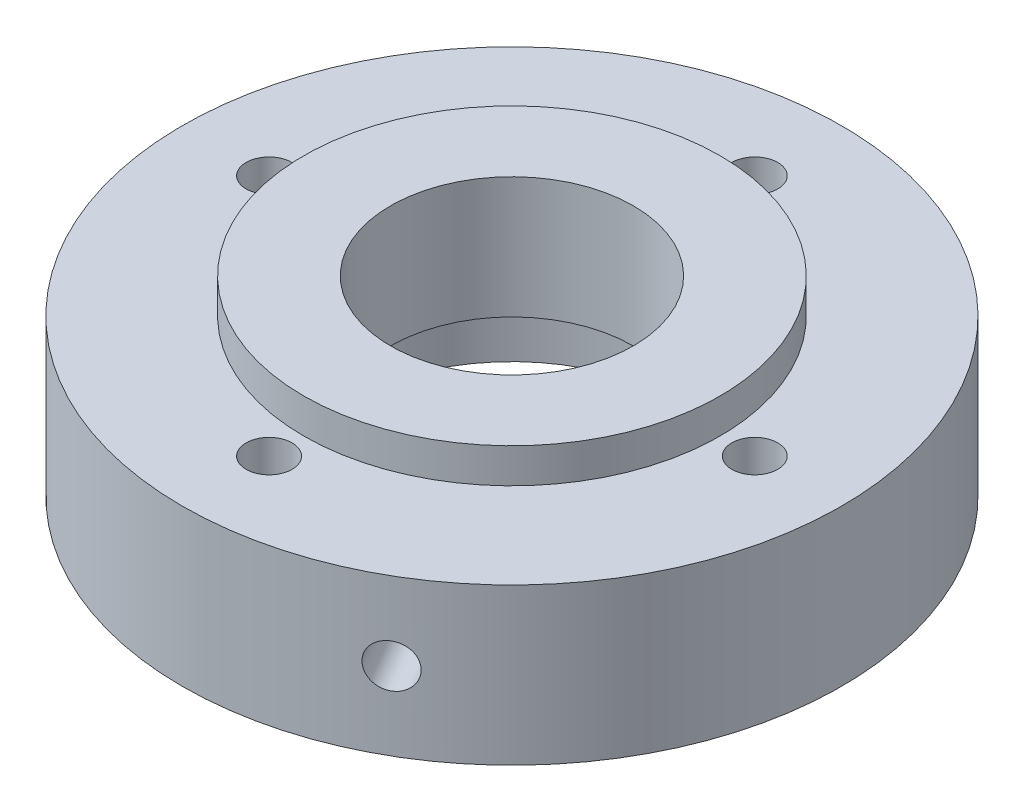
ISO-10303-21;
HEADER;
FILE_DESCRIPTION(('STEP AP214'),'2;1');
FILE_NAME('part.step','',(''),(''),'','','');
FILE_SCHEMA(('AUTOMOTIVE_DESIGN { 1 0 10303 214 1 1 1 1 }'));
ENDSEC;
DATA;
#1=APPLICATION_CONTEXT('core data for automotive mechanical design processes');
#2=APPLICATION_PROTOCOL_DEFINITION('international standard','automotive_design',2000,#1);
#3=PRODUCT_CONTEXT('',#1,'mechanical');
#4=PRODUCT('Part','Part','',(#3));
#5=PRODUCT_RELATED_PRODUCT_CATEGORY('part','',(#4));
#6=PRODUCT_DEFINITION_FORMATION('','',#4);
#7=PRODUCT_DEFINITION_CONTEXT('part definition',#1,'design');
#8=PRODUCT_DEFINITION('design','',#6,#7);
#9=PRODUCT_DEFINITION_SHAPE('','',#8);
#10=(LENGTH_UNIT() NAMED_UNIT(*) SI_UNIT(.MILLI.,.METRE.));
#11=(NAMED_UNIT(*) PLANE_ANGLE_UNIT() SI_UNIT($,.RADIAN.));
#12=(NAMED_UNIT(*) SI_UNIT($,.STERADIAN.) SOLID_ANGLE_UNIT());
#13=UNCERTAINTY_MEASURE_WITH_UNIT(LENGTH_MEASURE(1.E-05),#10,'distance_accuracy_value','');
#14=(GEOMETRIC_REPRESENTATION_CONTEXT(3) GLOBAL_UNCERTAINTY_ASSIGNED_CONTEXT((#13)) GLOBAL_UNIT_ASSIGNED_CONTEXT((#10,
#11,#12)) REPRESENTATION_CONTEXT('',''));
#15=CARTESIAN_POINT('',(0.,0.,0.));
#16=DIRECTION('',(0.,0.,1.));
#17=DIRECTION('',(1.,0.,0.));
#18=AXIS2_PLACEMENT_3D('',#15,#16,#17);
#19=CARTESIAN_POINT('',(0.,9.,0.));
#20=DIRECTION('',(0.,-1.,0.));
#21=DIRECTION('',(0.,0.,-1.));
#22=AXIS2_PLACEMENT_3D('',#19,#20,#21);
#23=CYLINDRICAL_SURFACE('',#22,38.);
#24=CARTESIAN_POINT('',(21.123900499108,0.,31.5876689184844));
#25=CARTESIAN_POINT('',(21.1238957091237,-0.14026296821929,31.587672954066));
#26=CARTESIAN_POINT('',(21.1140367111997,-0.280623770964307,31.594272124677));
#27=CARTESIAN_POINT('',(21.0748168683031,-0.557468570772763,31.6204463654553));
#28=CARTESIAN_POINT('',(21.0454334075926,-0.693947880391754,31.6400364833519));
#29=CARTESIAN_POINT('',(20.967916595861,-0.95897955673141,31.6914598000946));
#30=CARTESIAN_POINT('',(20.9197932437121,-1.08753610842819,31.7232864698813));
#31=CARTESIAN_POINT('',(20.8060316775886,-1.33312465995972,31.7980133802452));
#32=CARTESIAN_POINT('',(20.7403974370897,-1.4501592660541,31.8409111085659));
#33=CARTESIAN_POINT('',(20.5931762627847,-1.66960814521729,31.9363237417059));
#34=CARTESIAN_POINT('',(20.5115662158887,-1.77200085914129,31.9888525733152));
#35=CARTESIAN_POINT('',(20.3345586484823,-1.95907477171309,32.1016621974415));
#36=CARTESIAN_POINT('',(20.2391605494445,-2.0437552268142,32.1619433152218));
#37=CARTESIAN_POINT('',(20.0369910004709,-2.19306785872995,32.288282567244));
#38=CARTESIAN_POINT('',(19.9302094863448,-2.25768209399902,32.3543458041241));
#39=CARTESIAN_POINT('',(19.7082088944471,-2.36491326725031,32.4900509335556));
#40=CARTESIAN_POINT('',(19.5929899149586,-2.40753046141693,32.559692784419));
#41=CARTESIAN_POINT('',(19.3574500570501,-2.46949770266854,32.7002737038991));
#42=CARTESIAN_POINT('',(19.2371368803516,-2.48888166021506,32.7712107281016));
#43=CARTESIAN_POINT('',(18.9946226048038,-2.50393692466989,32.9123683968928));
#44=CARTESIAN_POINT('',(18.8724215291774,-2.49960852303035,32.9825890502759));
#45=CARTESIAN_POINT('',(18.629812232287,-2.46738987486286,33.1202283097107));
#46=CARTESIAN_POINT('',(18.5094015290169,-2.43953610408451,33.1876510841454));
#47=CARTESIAN_POINT('',(18.273667513676,-2.36111400348179,33.3180316189365));
#48=CARTESIAN_POINT('',(18.1583442342758,-2.31054552781078,33.3809893506207));
#49=CARTESIAN_POINT('',(17.9360874792135,-2.18808825789193,33.5009364538799));
#50=CARTESIAN_POINT('',(17.8291605790289,-2.11618296057238,33.5579211592496));
#51=CARTESIAN_POINT('',(17.6269807914162,-1.95310517722637,33.6645604903366));
#52=CARTESIAN_POINT('',(17.531728050049,-1.86193245017493,33.7142150243444));
#53=CARTESIAN_POINT('',(17.3556053972048,-1.6627019182125,33.8052189562838));
#54=CARTESIAN_POINT('',(17.2747630785516,-1.55461244874809,33.8465524403759));
#55=CARTESIAN_POINT('',(17.1301682937497,-1.32472755050962,33.9199636076438));
#56=CARTESIAN_POINT('',(17.0664158352165,-1.20293211562793,33.952041286695));
#57=CARTESIAN_POINT('',(16.957985484699,-0.949072071377019,34.0063291677514));
#58=CARTESIAN_POINT('',(16.9133088240632,-0.817006799736989,34.0285387327707));
#59=CARTESIAN_POINT('',(16.8444496087952,-0.546365405699918,34.0626776289473));
#60=CARTESIAN_POINT('',(16.820266786872,-0.407789368244477,34.0746070941829));
#61=CARTESIAN_POINT('',(16.7931920702844,-0.128338078964031,34.0879587586434));
#62=CARTESIAN_POINT('',(16.7902603680609,0.0125323783636798,34.0894006032779));
#63=CARTESIAN_POINT('',(16.8056762304921,0.292818040330734,34.081803318164));
#64=CARTESIAN_POINT('',(16.8240236722807,0.432233253367982,34.0727642489327));
#65=CARTESIAN_POINT('',(16.881387081484,0.70552541036977,34.0443795985637));
#66=CARTESIAN_POINT('',(16.920384723914,0.839407151357643,34.0250431552276));
#67=CARTESIAN_POINT('',(17.0178070267663,1.09798008966523,33.9764210990002));
#68=CARTESIAN_POINT('',(17.0762318823767,1.22267119462979,33.9471353861469));
#69=CARTESIAN_POINT('',(17.2107892564278,1.45952670684333,33.8791145571879));
#70=CARTESIAN_POINT('',(17.2869479539057,1.57167222814922,33.8403654668937));
#71=CARTESIAN_POINT('',(17.45458149206,1.78006283557162,33.7542062957108));
#72=CARTESIAN_POINT('',(17.5460564984008,1.87630774968148,33.7067961211417));
#73=CARTESIAN_POINT('',(17.7416982345965,2.05031494761945,33.6042309536316));
#74=CARTESIAN_POINT('',(17.8458842859506,2.12804855025184,33.5490641502799));
#75=CARTESIAN_POINT('',(18.0637061593128,2.26263021792935,33.4322863441705));
#76=CARTESIAN_POINT('',(18.1773419179329,2.3194784230582,33.3706753846389));
#77=CARTESIAN_POINT('',(18.4105992907013,2.41062578245923,33.2425557196137));
#78=CARTESIAN_POINT('',(18.5302160183662,2.44494303087561,33.176050992058));
#79=CARTESIAN_POINT('',(18.77202332052,2.49011354081496,33.0398303379182));
#80=CARTESIAN_POINT('',(18.8942138664263,2.50096706276853,32.9701144469845));
#81=CARTESIAN_POINT('',(19.1374242590965,2.49889944252103,32.8295398192453));
#82=CARTESIAN_POINT('',(19.258445880915,2.48602315917565,32.7586834892885));
#83=CARTESIAN_POINT('',(19.4961515734082,2.43695452332046,32.6177738646721));
#84=CARTESIAN_POINT('',(19.6128356366526,2.40076213087149,32.5477205713883));
#85=CARTESIAN_POINT('',(19.8386569858294,2.30609897011035,32.4105716618428));
#86=CARTESIAN_POINT('',(19.9477943666864,2.2476284820792,32.3434760083829));
#87=CARTESIAN_POINT('',(20.1555911399982,2.1100749002662,32.2143931549603));
#88=CARTESIAN_POINT('',(20.2542507892874,2.03099231190029,32.1524058297887));
#89=CARTESIAN_POINT('',(20.4386670176825,1.85429296810048,32.0354936565859));
#90=CARTESIAN_POINT('',(20.5244004228226,1.75664361852911,31.9805815178681));
#91=CARTESIAN_POINT('',(20.6805510807337,1.5456295694054,31.8798285309556));
#92=CARTESIAN_POINT('',(20.7509645857459,1.43226103549673,31.8339899026911));
#93=CARTESIAN_POINT('',(20.8747236923557,1.19288481911541,31.7529747632888));
#94=CARTESIAN_POINT('',(20.9280465194288,1.06686056310857,31.7178124823886));
#95=CARTESIAN_POINT('',(21.0160861318739,0.805961436994182,31.659547325594));
#96=CARTESIAN_POINT('',(21.0508246541216,0.671097114810736,31.6364303618878));
#97=CARTESIAN_POINT('',(21.0918211256234,0.44617637840564,31.6091035052925));
#98=CARTESIAN_POINT('',(21.1038367830818,0.357572910700806,31.6010785819328));
#99=CARTESIAN_POINT('',(21.1198779949323,0.179326293259485,31.5903600025264));
#100=CARTESIAN_POINT('',(21.1239035617899,0.0896831451452361,31.5876663381622));
#101=CARTESIAN_POINT('',(21.123900499108,0.,31.5876689184844));
#102=B_SPLINE_CURVE_WITH_KNOTS('',3,(#24,#25,#26,#27,#28,#29,#30,#31,#32,#33,#34,#35,#36,#37,
#38,#39,#40,#41,#42,#43,#44,#45,#46,#47,#48,#49,#50,#51,#52,#53,#54,#55,#56,#57,#58,#59,#60,#61,
#62,#63,#64,#65,#66,#67,#68,#69,#70,#71,#72,#73,#74,#75,#76,#77,#78,#79,#80,#81,#82,#83,#84,#85,
#86,#87,#88,#89,#90,#91,#92,#93,#94,#95,#96,#97,#98,#99,#100,#101),.UNSPECIFIED.,.T.,.F.,(4,2,2,
2,2,2,2,2,2,2,2,2,2,2,2,2,2,2,2,2,2,2,2,2,2,2,2,2,2,2,2,2,2,2,2,2,2,2,4),(0.,0.420461498480437,
0.841410880410043,1.26213596730298,1.68276566662256,2.10400847286644,2.52526895900485,
2.94690502397213,3.36853617832339,3.78955118149476,4.21056100991944,4.63091926439621,
5.05128021794911,5.47196715304152,5.89265935100819,6.31414862675714,6.7356380903302,
7.15715475706393,7.57866592607824,7.99938731660346,8.42010627789137,8.84045251737814,
9.26080298027826,9.68177795124712,10.1027574758629,10.5243850778361,10.946009851793,
11.3672956121168,11.7885766964458,12.2090622072308,12.6295484382853,13.0500293793716,
13.4705000110872,13.8917157147232,14.3130343462041,14.7349121022704,15.1562953299902,
15.4251358436648,15.6939759379172),.UNSPECIFIED.);
#103=CARTESIAN_POINT('',(21.123900499108,0.,31.5876689184844));
#104=VERTEX_POINT('',#103);
#105=EDGE_CURVE('E70',#104,#104,#102,.T.);
#106=ORIENTED_EDGE('',*,*,#105,.T.);
#107=EDGE_LOOP('',(#106));
#108=FACE_BOUND('',#107,.T.);
#109=CARTESIAN_POINT('',(0.,9.,0.));
#110=DIRECTION('',(0.,1.,0.));
#111=DIRECTION('',(0.,0.,1.));
#112=AXIS2_PLACEMENT_3D('',#109,#110,#111);
#113=CIRCLE('',#112,38.);
#114=CARTESIAN_POINT('',(0.,9.,38.));
#115=VERTEX_POINT('',#114);
#116=EDGE_CURVE('E78',#115,#115,#113,.T.);
#117=ORIENTED_EDGE('',*,*,#116,.F.);
#118=EDGE_LOOP('',(#117));
#119=FACE_BOUND('',#118,.T.);
#120=CARTESIAN_POINT('',(0.,-9.,0.));
#121=DIRECTION('',(0.,1.,0.));
#122=DIRECTION('',(0.,0.,1.));
#123=AXIS2_PLACEMENT_3D('',#120,#121,#122);
#124=CIRCLE('',#123,38.);
#125=CARTESIAN_POINT('',(0.,-9.,38.));
#126=VERTEX_POINT('',#125);
#127=EDGE_CURVE('E81',#126,#126,#124,.T.);
#128=ORIENTED_EDGE('',*,*,#127,.T.);
#129=EDGE_LOOP('',(#128));
#130=FACE_BOUND('',#129,.T.);
#131=ADVANCED_FACE('F39',(#108,#119,#130),#23,.T.);
#132=CARTESIAN_POINT('',(0.,9.,0.));
#133=DIRECTION('',(0.,1.,0.));
#134=DIRECTION('',(0.,0.,1.));
#135=AXIS2_PLACEMENT_3D('',#132,#133,#134);
#136=PLANE('',#135);
#137=CARTESIAN_POINT('',(0.,9.,28.));
#138=DIRECTION('',(0.,-1.,0.));
#139=DIRECTION('',(0.,0.,-1.));
#140=AXIS2_PLACEMENT_3D('',#137,#138,#139);
#141=CIRCLE('',#140,2.65000000000001);
#142=CARTESIAN_POINT('',(0.,9.,25.35));
#143=VERTEX_POINT('',#142);
#144=EDGE_CURVE('E204',#143,#143,#141,.T.);
#145=ORIENTED_EDGE('',*,*,#144,.T.);
#146=EDGE_LOOP('',(#145));
#147=FACE_BOUND('',#146,.T.);
#148=CARTESIAN_POINT('',(28.,9.,0.));
#149=DIRECTION('',(0.,-1.,0.));
#150=DIRECTION('',(0.,0.,-1.));
#151=AXIS2_PLACEMENT_3D('',#148,#149,#150);
#152=CIRCLE('',#151,2.65000000000001);
#153=CARTESIAN_POINT('',(28.,9.,-2.65000000000001));
#154=VERTEX_POINT('',#153);
#155=EDGE_CURVE('E213',#154,#154,#152,.T.);
#156=ORIENTED_EDGE('',*,*,#155,.T.);
#157=EDGE_LOOP('',(#156));
#158=FACE_BOUND('',#157,.T.);
#159=CARTESIAN_POINT('',(0.,9.,-28.));
#160=DIRECTION('',(0.,-1.,0.));
#161=DIRECTION('',(0.,0.,-1.));
#162=AXIS2_PLACEMENT_3D('',#159,#160,#161);
#163=CIRCLE('',#162,2.65000000000001);
#164=CARTESIAN_POINT('',(0.,9.,-30.65));
#165=VERTEX_POINT('',#164);
#166=EDGE_CURVE('E227',#165,#165,#163,.T.);
#167=ORIENTED_EDGE('',*,*,#166,.T.);
#168=EDGE_LOOP('',(#167));
#169=FACE_BOUND('',#168,.T.);
#170=CARTESIAN_POINT('',(-28.,9.,0.));
#171=DIRECTION('',(0.,-1.,0.));
#172=DIRECTION('',(0.,0.,-1.));
#173=AXIS2_PLACEMENT_3D('',#170,#171,#172);
#174=CIRCLE('',#173,2.65000000000001);
#175=CARTESIAN_POINT('',(-28.,9.,-2.65000000000001));
#176=VERTEX_POINT('',#175);
#177=EDGE_CURVE('E237',#176,#176,#174,.T.);
#178=ORIENTED_EDGE('',*,*,#177,.T.);
#179=EDGE_LOOP('',(#178));
#180=FACE_BOUND('',#179,.T.);
#181=CARTESIAN_POINT('',(0.,9.,0.));
#182=DIRECTION('',(0.,1.,0.));
#183=DIRECTION('',(0.,0.,1.));
#184=AXIS2_PLACEMENT_3D('',#181,#182,#183);
#185=CIRCLE('',#184,24.);
#186=CARTESIAN_POINT('',(0.,9.,24.));
#187=VERTEX_POINT('',#186);
#188=EDGE_CURVE('E242',#187,#187,#185,.F.);
#189=ORIENTED_EDGE('',*,*,#188,.T.);
#190=EDGE_LOOP('',(#189));
#191=FACE_BOUND('',#190,.T.);
#192=ORIENTED_EDGE('',*,*,#116,.T.);
#193=EDGE_LOOP('',(#192));
#194=FACE_BOUND('',#193,.T.);
#195=ADVANCED_FACE('F111',(#147,#158,#169,#180,#191,#194),#136,.T.);
#196=CARTESIAN_POINT('',(0.,-9.,0.));
#197=DIRECTION('',(0.,1.,0.));
#198=DIRECTION('',(0.,0.,1.));
#199=AXIS2_PLACEMENT_3D('',#196,#197,#198);
#200=PLANE('',#199);
#201=CARTESIAN_POINT('',(0.,-9.,0.));
#202=DIRECTION('',(0.,1.,0.));
#203=DIRECTION('',(0.,0.,1.));
#204=AXIS2_PLACEMENT_3D('',#201,#202,#203);
#205=CIRCLE('',#204,19.);
#206=CARTESIAN_POINT('',(0.,-9.,19.));
#207=VERTEX_POINT('',#206);
#208=EDGE_CURVE('E86',#207,#207,#205,.T.);
#209=ORIENTED_EDGE('',*,*,#208,.T.);
#210=EDGE_LOOP('',(#209));
#211=FACE_BOUND('',#210,.T.);
#212=CARTESIAN_POINT('',(0.,-9.,28.));
#213=DIRECTION('',(0.,-1.,0.));
#214=DIRECTION('',(0.,0.,-1.));
#215=AXIS2_PLACEMENT_3D('',#212,#213,#214);
#216=CIRCLE('',#215,3.90000000000001);
#217=CARTESIAN_POINT('',(0.,-9.,24.1));
#218=VERTEX_POINT('',#217);
#219=EDGE_CURVE('E194',#218,#218,#216,.T.);
#220=ORIENTED_EDGE('',*,*,#219,.F.);
#221=EDGE_LOOP('',(#220));
#222=FACE_BOUND('',#221,.T.);
#223=CARTESIAN_POINT('',(28.,-9.,0.));
#224=DIRECTION('',(0.,-1.,0.));
#225=DIRECTION('',(0.,0.,-1.));
#226=AXIS2_PLACEMENT_3D('',#223,#224,#225);
#227=CIRCLE('',#226,3.90000000000001);
#228=CARTESIAN_POINT('',(28.,-9.,-3.90000000000001));
#229=VERTEX_POINT('',#228);
#230=EDGE_CURVE('E207',#229,#229,#227,.T.);
#231=ORIENTED_EDGE('',*,*,#230,.F.);
#232=EDGE_LOOP('',(#231));
#233=FACE_BOUND('',#232,.T.);
#234=CARTESIAN_POINT('',(0.,-9.,-28.));
#235=DIRECTION('',(0.,-1.,0.));
#236=DIRECTION('',(0.,0.,-1.));
#237=AXIS2_PLACEMENT_3D('',#234,#235,#236);
#238=CIRCLE('',#237,3.90000000000001);
#239=CARTESIAN_POINT('',(0.,-9.,-31.9));
#240=VERTEX_POINT('',#239);
#241=EDGE_CURVE('E220',#240,#240,#238,.T.);
#242=ORIENTED_EDGE('',*,*,#241,.F.);
#243=EDGE_LOOP('',(#242));
#244=FACE_BOUND('',#243,.T.);
#245=CARTESIAN_POINT('',(-28.,-9.,0.));
#246=DIRECTION('',(0.,-1.,0.));
#247=DIRECTION('',(0.,0.,-1.));
#248=AXIS2_PLACEMENT_3D('',#245,#246,#247);
#249=CIRCLE('',#248,3.90000000000001);
#250=CARTESIAN_POINT('',(-28.,-9.,-3.90000000000001));
#251=VERTEX_POINT('',#250);
#252=EDGE_CURVE('E229',#251,#251,#249,.T.);
#253=ORIENTED_EDGE('',*,*,#252,.F.);
#254=EDGE_LOOP('',(#253));
#255=FACE_BOUND('',#254,.T.);
#256=ORIENTED_EDGE('',*,*,#127,.F.);
#257=EDGE_LOOP('',(#256));
#258=FACE_BOUND('',#257,.T.);
#259=ADVANCED_FACE('F113',(#211,#222,#233,#244,#255,#258),#200,.F.);
#260=CARTESIAN_POINT('',(0.,13.,0.));
#261=DIRECTION('',(0.,-1.,0.));
#262=DIRECTION('',(0.,0.,-1.));
#263=AXIS2_PLACEMENT_3D('',#260,#261,#262);
#264=CYLINDRICAL_SURFACE('',#263,24.);
#265=ORIENTED_EDGE('',*,*,#188,.F.);
#266=EDGE_LOOP('',(#265));
#267=FACE_BOUND('',#266,.T.);
#268=CARTESIAN_POINT('',(0.,13.,0.));
#269=DIRECTION('',(0.,1.,0.));
#270=DIRECTION('',(0.,0.,1.));
#271=AXIS2_PLACEMENT_3D('',#268,#269,#270);
#272=CIRCLE('',#271,24.);
#273=CARTESIAN_POINT('',(0.,13.,24.));
#274=VERTEX_POINT('',#273);
#275=EDGE_CURVE('E245',#274,#274,#272,.T.);
#276=ORIENTED_EDGE('',*,*,#275,.F.);
#277=EDGE_LOOP('',(#276));
#278=FACE_BOUND('',#277,.T.);
#279=ADVANCED_FACE('F116',(#267,#278),#264,.T.);
#280=CARTESIAN_POINT('',(0.,13.,0.));
#281=DIRECTION('',(0.,1.,0.));
#282=DIRECTION('',(0.,0.,1.));
#283=AXIS2_PLACEMENT_3D('',#280,#281,#282);
#284=PLANE('',#283);
#285=CARTESIAN_POINT('',(0.,13.,0.));
#286=DIRECTION('',(0.,1.,0.));
#287=DIRECTION('',(0.,0.,1.));
#288=AXIS2_PLACEMENT_3D('',#285,#286,#287);
#289=CIRCLE('',#288,14.);
#290=CARTESIAN_POINT('',(0.,13.,-14.));
#291=VERTEX_POINT('',#290);
#292=EDGE_CURVE('E102',#291,#291,#289,.F.);
#293=ORIENTED_EDGE('',*,*,#292,.T.);
#294=EDGE_LOOP('',(#293));
#295=FACE_BOUND('',#294,.T.);
#296=ORIENTED_EDGE('',*,*,#275,.T.);
#297=EDGE_LOOP('',(#296));
#298=FACE_BOUND('',#297,.T.);
#299=ADVANCED_FACE('F124',(#295,#298),#284,.T.);
#300=CARTESIAN_POINT('',(-28.,-9.,0.));
#301=DIRECTION('',(0.,-1.,0.));
#302=DIRECTION('',(0.,0.,-1.));
#303=AXIS2_PLACEMENT_3D('',#300,#301,#302);
#304=CYLINDRICAL_SURFACE('',#303,2.65000000000001);
#305=ORIENTED_EDGE('',*,*,#177,.F.);
#306=EDGE_LOOP('',(#305));
#307=FACE_BOUND('',#306,.T.);
#308=CARTESIAN_POINT('',(-28.,-5.,0.));
#309=DIRECTION('',(0.,-1.,0.));
#310=DIRECTION('',(0.,0.,-1.));
#311=AXIS2_PLACEMENT_3D('',#308,#309,#310);
#312=CIRCLE('',#311,2.65000000000001);
#313=CARTESIAN_POINT('',(-28.,-5.,-2.65000000000001));
#314=VERTEX_POINT('',#313);
#315=EDGE_CURVE('E236',#314,#314,#312,.T.);
#316=ORIENTED_EDGE('',*,*,#315,.T.);
#317=EDGE_LOOP('',(#316));
#318=FACE_BOUND('',#317,.T.);
#319=ADVANCED_FACE('F130',(#307,#318),#304,.F.);
#320=CARTESIAN_POINT('',(-25.35,-5.,0.));
#321=DIRECTION('',(0.,1.,0.));
#322=DIRECTION('',(0.,0.,1.));
#323=AXIS2_PLACEMENT_3D('',#320,#321,#322);
#324=PLANE('',#323);
#325=ORIENTED_EDGE('',*,*,#315,.F.);
#326=EDGE_LOOP('',(#325));
#327=FACE_BOUND('',#326,.T.);
#328=CARTESIAN_POINT('',(-28.,-5.,0.));
#329=DIRECTION('',(0.,-1.,0.));
#330=DIRECTION('',(0.,0.,-1.));
#331=AXIS2_PLACEMENT_3D('',#328,#329,#330);
#332=CIRCLE('',#331,3.90000000000001);
#333=CARTESIAN_POINT('',(-28.,-5.,-3.90000000000001));
#334=VERTEX_POINT('',#333);
#335=EDGE_CURVE('E231',#334,#334,#332,.T.);
#336=ORIENTED_EDGE('',*,*,#335,.T.);
#337=EDGE_LOOP('',(#336));
#338=FACE_BOUND('',#337,.T.);
#339=ADVANCED_FACE('F134',(#327,#338),#324,.F.);
#340=CARTESIAN_POINT('',(-28.,-9.,0.));
#341=DIRECTION('',(0.,-1.,0.));
#342=DIRECTION('',(0.,0.,-1.));
#343=AXIS2_PLACEMENT_3D('',#340,#341,#342);
#344=CYLINDRICAL_SURFACE('',#343,3.90000000000001);
#345=ORIENTED_EDGE('',*,*,#335,.F.);
#346=EDGE_LOOP('',(#345));
#347=FACE_BOUND('',#346,.T.);
#348=ORIENTED_EDGE('',*,*,#252,.T.);
#349=EDGE_LOOP('',(#348));
#350=FACE_BOUND('',#349,.T.);
#351=ADVANCED_FACE('F132',(#347,#350),#344,.F.);
#352=CARTESIAN_POINT('',(0.,-9.,-28.));
#353=DIRECTION('',(0.,-1.,0.));
#354=DIRECTION('',(0.,0.,-1.));
#355=AXIS2_PLACEMENT_3D('',#352,#353,#354);
#356=CYLINDRICAL_SURFACE('',#355,2.65000000000001);
#357=ORIENTED_EDGE('',*,*,#166,.F.);
#358=EDGE_LOOP('',(#357));
#359=FACE_BOUND('',#358,.T.);
#360=CARTESIAN_POINT('',(0.,-5.,-28.));
#361=DIRECTION('',(0.,-1.,0.));
#362=DIRECTION('',(0.,0.,-1.));
#363=AXIS2_PLACEMENT_3D('',#360,#361,#362);
#364=CIRCLE('',#363,2.65000000000001);
#365=CARTESIAN_POINT('',(0.,-5.,-30.65));
#366=VERTEX_POINT('',#365);
#367=EDGE_CURVE('E221',#366,#366,#364,.T.);
#368=ORIENTED_EDGE('',*,*,#367,.T.);
#369=EDGE_LOOP('',(#368));
#370=FACE_BOUND('',#369,.T.);
#371=ADVANCED_FACE('F136',(#359,#370),#356,.F.);
#372=CARTESIAN_POINT('',(2.65000000000001,-5.,-28.));
#373=DIRECTION('',(0.,1.,0.));
#374=DIRECTION('',(0.,0.,1.));
#375=AXIS2_PLACEMENT_3D('',#372,#373,#374);
#376=PLANE('',#375);
#377=ORIENTED_EDGE('',*,*,#367,.F.);
#378=EDGE_LOOP('',(#377));
#379=FACE_BOUND('',#378,.T.);
#380=CARTESIAN_POINT('',(0.,-5.,-28.));
#381=DIRECTION('',(0.,-1.,0.));
#382=DIRECTION('',(0.,0.,-1.));
#383=AXIS2_PLACEMENT_3D('',#380,#381,#382);
#384=CIRCLE('',#383,3.90000000000001);
#385=CARTESIAN_POINT('',(0.,-5.,-31.9));
#386=VERTEX_POINT('',#385);
#387=EDGE_CURVE('E222',#386,#386,#384,.T.);
#388=ORIENTED_EDGE('',*,*,#387,.T.);
#389=EDGE_LOOP('',(#388));
#390=FACE_BOUND('',#389,.T.);
#391=ADVANCED_FACE('F141',(#379,#390),#376,.F.);
#392=CARTESIAN_POINT('',(0.,-9.,-28.));
#393=DIRECTION('',(0.,-1.,0.));
#394=DIRECTION('',(0.,0.,-1.));
#395=AXIS2_PLACEMENT_3D('',#392,#393,#394);
#396=CYLINDRICAL_SURFACE('',#395,3.90000000000001);
#397=ORIENTED_EDGE('',*,*,#387,.F.);
#398=EDGE_LOOP('',(#397));
#399=FACE_BOUND('',#398,.T.);
#400=ORIENTED_EDGE('',*,*,#241,.T.);
#401=EDGE_LOOP('',(#400));
#402=FACE_BOUND('',#401,.T.);
#403=ADVANCED_FACE('F150',(#399,#402),#396,.F.);
#404=CARTESIAN_POINT('',(28.,-9.,0.));
#405=DIRECTION('',(0.,-1.,0.));
#406=DIRECTION('',(0.,0.,-1.));
#407=AXIS2_PLACEMENT_3D('',#404,#405,#406);
#408=CYLINDRICAL_SURFACE('',#407,2.65000000000001);
#409=ORIENTED_EDGE('',*,*,#155,.F.);
#410=EDGE_LOOP('',(#409));
#411=FACE_BOUND('',#410,.T.);
#412=CARTESIAN_POINT('',(28.,-5.,0.));
#413=DIRECTION('',(0.,-1.,0.));
#414=DIRECTION('',(0.,0.,-1.));
#415=AXIS2_PLACEMENT_3D('',#412,#413,#414);
#416=CIRCLE('',#415,2.65000000000001);
#417=CARTESIAN_POINT('',(28.,-5.,-2.65000000000001));
#418=VERTEX_POINT('',#417);
#419=EDGE_CURVE('E215',#418,#418,#416,.T.);
#420=ORIENTED_EDGE('',*,*,#419,.T.);
#421=EDGE_LOOP('',(#420));
#422=FACE_BOUND('',#421,.T.);
#423=ADVANCED_FACE('F154',(#411,#422),#408,.F.);
#424=CARTESIAN_POINT('',(30.65,-5.,0.));
#425=DIRECTION('',(0.,1.,0.));
#426=DIRECTION('',(0.,0.,1.));
#427=AXIS2_PLACEMENT_3D('',#424,#425,#426);
#428=PLANE('',#427);
#429=ORIENTED_EDGE('',*,*,#419,.F.);
#430=EDGE_LOOP('',(#429));
#431=FACE_BOUND('',#430,.T.);
#432=CARTESIAN_POINT('',(28.,-5.,0.));
#433=DIRECTION('',(0.,-1.,0.));
#434=DIRECTION('',(0.,0.,-1.));
#435=AXIS2_PLACEMENT_3D('',#432,#433,#434);
#436=CIRCLE('',#435,3.90000000000001);
#437=CARTESIAN_POINT('',(28.,-5.,-3.90000000000001));
#438=VERTEX_POINT('',#437);
#439=EDGE_CURVE('E209',#438,#438,#436,.T.);
#440=ORIENTED_EDGE('',*,*,#439,.T.);
#441=EDGE_LOOP('',(#440));
#442=FACE_BOUND('',#441,.T.);
#443=ADVANCED_FACE('F152',(#431,#442),#428,.F.);
#444=CARTESIAN_POINT('',(28.,-9.,0.));
#445=DIRECTION('',(0.,-1.,0.));
#446=DIRECTION('',(0.,0.,-1.));
#447=AXIS2_PLACEMENT_3D('',#444,#445,#446);
#448=CYLINDRICAL_SURFACE('',#447,3.90000000000001);
#449=ORIENTED_EDGE('',*,*,#439,.F.);
#450=EDGE_LOOP('',(#449));
#451=FACE_BOUND('',#450,.T.);
#452=ORIENTED_EDGE('',*,*,#230,.T.);
#453=EDGE_LOOP('',(#452));
#454=FACE_BOUND('',#453,.T.);
#455=ADVANCED_FACE('F156',(#451,#454),#448,.F.);
#456=CARTESIAN_POINT('',(0.,-9.,28.));
#457=DIRECTION('',(0.,-1.,0.));
#458=DIRECTION('',(0.,0.,-1.));
#459=AXIS2_PLACEMENT_3D('',#456,#457,#458);
#460=CYLINDRICAL_SURFACE('',#459,2.65000000000001);
#461=ORIENTED_EDGE('',*,*,#144,.F.);
#462=EDGE_LOOP('',(#461));
#463=FACE_BOUND('',#462,.T.);
#464=CARTESIAN_POINT('',(0.,-5.,28.));
#465=DIRECTION('',(0.,-1.,0.));
#466=DIRECTION('',(0.,0.,-1.));
#467=AXIS2_PLACEMENT_3D('',#464,#465,#466);
#468=CIRCLE('',#467,2.65000000000001);
#469=CARTESIAN_POINT('',(0.,-5.,25.35));
#470=VERTEX_POINT('',#469);
#471=EDGE_CURVE('E197',#470,#470,#468,.T.);
#472=ORIENTED_EDGE('',*,*,#471,.T.);
#473=EDGE_LOOP('',(#472));
#474=FACE_BOUND('',#473,.T.);
#475=ADVANCED_FACE('F161',(#463,#474),#460,.F.);
#476=CARTESIAN_POINT('',(2.65000000000001,-5.,28.));
#477=DIRECTION('',(0.,1.,0.));
#478=DIRECTION('',(0.,0.,1.));
#479=AXIS2_PLACEMENT_3D('',#476,#477,#478);
#480=PLANE('',#479);
#481=ORIENTED_EDGE('',*,*,#471,.F.);
#482=EDGE_LOOP('',(#481));
#483=FACE_BOUND('',#482,.T.);
#484=CARTESIAN_POINT('',(0.,-5.,28.));
#485=DIRECTION('',(0.,-1.,0.));
#486=DIRECTION('',(0.,0.,-1.));
#487=AXIS2_PLACEMENT_3D('',#484,#485,#486);
#488=CIRCLE('',#487,3.90000000000001);
#489=CARTESIAN_POINT('',(0.,-5.,24.1));
#490=VERTEX_POINT('',#489);
#491=EDGE_CURVE('E196',#490,#490,#488,.T.);
#492=ORIENTED_EDGE('',*,*,#491,.T.);
#493=EDGE_LOOP('',(#492));
#494=FACE_BOUND('',#493,.T.);
#495=ADVANCED_FACE('F170',(#483,#494),#480,.F.);
#496=CARTESIAN_POINT('',(0.,-9.,28.));
#497=DIRECTION('',(0.,-1.,0.));
#498=DIRECTION('',(0.,0.,-1.));
#499=AXIS2_PLACEMENT_3D('',#496,#497,#498);
#500=CYLINDRICAL_SURFACE('',#499,3.90000000000001);
#501=ORIENTED_EDGE('',*,*,#491,.F.);
#502=EDGE_LOOP('',(#501));
#503=FACE_BOUND('',#502,.T.);
#504=ORIENTED_EDGE('',*,*,#219,.T.);
#505=EDGE_LOOP('',(#504));
#506=FACE_BOUND('',#505,.T.);
#507=ADVANCED_FACE('F171',(#503,#506),#500,.F.);
#508=CARTESIAN_POINT('',(0.,-1.,0.));
#509=DIRECTION('',(0.,-1.,0.));
#510=DIRECTION('',(0.,0.,-1.));
#511=AXIS2_PLACEMENT_3D('',#508,#509,#510);
#512=CYLINDRICAL_SURFACE('',#511,19.);
#513=CARTESIAN_POINT('',(0.,-3.,0.));
#514=DIRECTION('',(0.,-1.,0.));
#515=DIRECTION('',(0.,0.,-1.));
#516=AXIS2_PLACEMENT_3D('',#513,#514,#515);
#517=CIRCLE('',#516,19.);
#518=CARTESIAN_POINT('',(0.,-3.,-19.));
#519=VERTEX_POINT('',#518);
#520=EDGE_CURVE('E63',#519,#519,#517,.F.);
#521=ORIENTED_EDGE('',*,*,#520,.T.);
#522=EDGE_LOOP('',(#521));
#523=FACE_BOUND('',#522,.T.);
#524=ORIENTED_EDGE('',*,*,#208,.F.);
#525=EDGE_LOOP('',(#524));
#526=FACE_BOUND('',#525,.T.);
#527=ADVANCED_FACE('F174',(#523,#526),#512,.F.);
#528=CARTESIAN_POINT('',(0.,-1.,0.));
#529=DIRECTION('',(0.,-1.,0.));
#530=DIRECTION('',(0.,0.,-1.));
#531=AXIS2_PLACEMENT_3D('',#528,#529,#530);
#532=PLANE('',#531);
#533=CARTESIAN_POINT('',(0.,-1.,0.));
#534=DIRECTION('',(0.,-1.,0.));
#535=DIRECTION('',(0.,0.,-1.));
#536=AXIS2_PLACEMENT_3D('',#533,#534,#535);
#537=CIRCLE('',#536,17.);
#538=CARTESIAN_POINT('',(0.,-1.,-17.));
#539=VERTEX_POINT('',#538);
#540=EDGE_CURVE('E76',#539,#539,#537,.T.);
#541=ORIENTED_EDGE('',*,*,#540,.T.);
#542=EDGE_LOOP('',(#541));
#543=FACE_BOUND('',#542,.T.);
#544=CARTESIAN_POINT('',(0.,-1.,0.));
#545=DIRECTION('',(0.,-1.,0.));
#546=DIRECTION('',(0.,0.,-1.));
#547=AXIS2_PLACEMENT_3D('',#544,#545,#546);
#548=CIRCLE('',#547,14.);
#549=CARTESIAN_POINT('',(0.,-0.999999999999999,-14.));
#550=VERTEX_POINT('',#549);
#551=EDGE_CURVE('E106',#550,#550,#548,.T.);
#552=ORIENTED_EDGE('',*,*,#551,.F.);
#553=EDGE_LOOP('',(#552));
#554=FACE_BOUND('',#553,.T.);
#555=ADVANCED_FACE('F177',(#543,#554),#532,.T.);
#556=CARTESIAN_POINT('',(0.,13.001,0.));
#557=DIRECTION('',(0.,-1.,0.));
#558=DIRECTION('',(0.,0.,-1.));
#559=AXIS2_PLACEMENT_3D('',#556,#557,#558);
#560=CYLINDRICAL_SURFACE('',#559,14.);
#561=CARTESIAN_POINT('',(0.,13.,-14.));
#562=CARTESIAN_POINT('',(0.,12.8541666666667,-14.));
#563=CARTESIAN_POINT('',(0.,12.7083333333333,-14.));
#564=CARTESIAN_POINT('',(0.,12.4166666666667,-14.));
#565=CARTESIAN_POINT('',(0.,12.2708333333333,-14.));
#566=CARTESIAN_POINT('',(0.,11.9791666666667,-14.));
#567=CARTESIAN_POINT('',(0.,11.8333333333333,-14.));
#568=CARTESIAN_POINT('',(0.,11.5416666666667,-14.));
#569=CARTESIAN_POINT('',(0.,11.3958333333333,-14.));
#570=CARTESIAN_POINT('',(0.,11.1041666666667,-14.));
#571=CARTESIAN_POINT('',(0.,10.9583333333333,-14.));
#572=CARTESIAN_POINT('',(0.,10.6666666666667,-14.));
#573=CARTESIAN_POINT('',(0.,10.5208333333333,-14.));
#574=CARTESIAN_POINT('',(0.,10.2291666666667,-14.));
#575=CARTESIAN_POINT('',(0.,10.0833333333333,-14.));
#576=CARTESIAN_POINT('',(0.,9.79166666666667,-14.));
#577=CARTESIAN_POINT('',(0.,9.64583333333333,-14.));
#578=CARTESIAN_POINT('',(0.,9.35416666666667,-14.));
#579=CARTESIAN_POINT('',(0.,9.20833333333333,-14.));
#580=CARTESIAN_POINT('',(0.,8.91666666666667,-14.));
#581=CARTESIAN_POINT('',(0.,8.77083333333333,-14.));
#582=CARTESIAN_POINT('',(0.,8.47916666666667,-14.));
#583=CARTESIAN_POINT('',(0.,8.33333333333333,-14.));
#584=CARTESIAN_POINT('',(0.,8.04166666666667,-14.));
#585=CARTESIAN_POINT('',(0.,7.89583333333333,-14.));
#586=CARTESIAN_POINT('',(0.,7.60416666666667,-14.));
#587=CARTESIAN_POINT('',(0.,7.45833333333333,-14.));
#588=CARTESIAN_POINT('',(0.,7.16666666666667,-14.));
#589=CARTESIAN_POINT('',(0.,7.02083333333333,-14.));
#590=CARTESIAN_POINT('',(0.,6.72916666666667,-14.));
#591=CARTESIAN_POINT('',(0.,6.58333333333333,-14.));
#592=CARTESIAN_POINT('',(0.,6.29166666666667,-14.));
#593=CARTESIAN_POINT('',(0.,6.14583333333333,-14.));
#594=CARTESIAN_POINT('',(0.,5.85416666666667,-14.));
#595=CARTESIAN_POINT('',(0.,5.70833333333333,-14.));
#596=CARTESIAN_POINT('',(0.,5.41666666666667,-14.));
#597=CARTESIAN_POINT('',(0.,5.27083333333333,-14.));
#598=CARTESIAN_POINT('',(0.,4.97916666666667,-14.));
#599=CARTESIAN_POINT('',(0.,4.83333333333333,-14.));
#600=CARTESIAN_POINT('',(0.,4.54166666666667,-14.));
#601=CARTESIAN_POINT('',(0.,4.39583333333334,-14.));
#602=CARTESIAN_POINT('',(0.,4.10416666666667,-14.));
#603=CARTESIAN_POINT('',(0.,3.95833333333334,-14.));
#604=CARTESIAN_POINT('',(0.,3.66666666666667,-14.));
#605=CARTESIAN_POINT('',(0.,3.52083333333333,-14.));
#606=CARTESIAN_POINT('',(0.,3.22916666666667,-14.));
#607=CARTESIAN_POINT('',(0.,3.08333333333333,-14.));
#608=CARTESIAN_POINT('',(0.,2.79166666666667,-14.));
#609=CARTESIAN_POINT('',(0.,2.64583333333333,-14.));
#610=CARTESIAN_POINT('',(0.,2.35416666666667,-14.));
#611=CARTESIAN_POINT('',(0.,2.20833333333333,-14.));
#612=CARTESIAN_POINT('',(0.,1.91666666666667,-14.));
#613=CARTESIAN_POINT('',(0.,1.77083333333333,-14.));
#614=CARTESIAN_POINT('',(0.,1.47916666666667,-14.));
#615=CARTESIAN_POINT('',(0.,1.33333333333334,-14.));
#616=CARTESIAN_POINT('',(0.,1.04166666666667,-14.));
#617=CARTESIAN_POINT('',(0.,0.895833333333336,-14.));
#618=CARTESIAN_POINT('',(0.,0.604166666666669,-14.));
#619=CARTESIAN_POINT('',(0.,0.458333333333335,-14.));
#620=CARTESIAN_POINT('',(0.,0.166666666666669,-14.));
#621=CARTESIAN_POINT('',(0.,0.020833333333335,-14.));
#622=CARTESIAN_POINT('',(0.,-0.270833333333332,-14.));
#623=CARTESIAN_POINT('',(0.,-0.416666666666665,-14.));
#624=CARTESIAN_POINT('',(0.,-0.708333333333332,-14.));
#625=CARTESIAN_POINT('',(0.,-0.854166666666666,-14.));
#626=CARTESIAN_POINT('',(0.,-0.999999999999999,-14.));
#627=B_SPLINE_CURVE_WITH_KNOTS('',3,(#561,#562,#563,#564,#565,#566,#567,#568,#569,#570,#571,
#572,#573,#574,#575,#576,#577,#578,#579,#580,#581,#582,#583,#584,#585,#586,#587,#588,#589,#590,
#591,#592,#593,#594,#595,#596,#597,#598,#599,#600,#601,#602,#603,#604,#605,#606,#607,#608,#609,
#610,#611,#612,#613,#614,#615,#616,#617,#618,#619,#620,#621,#622,#623,#624,#625,#626),
.UNSPECIFIED.,.F.,.F.,(4,2,2,2,2,2,2,2,2,2,2,2,2,2,2,2,2,2,2,2,2,2,2,2,2,2,2,2,2,2,2,2,4),(0.,
0.4375,0.875000000000001,1.3125,1.75,2.1875,2.625,3.0625,3.5,3.9375,4.375,4.8125,5.25,5.6875,
6.125,6.5625,7.,7.4375,7.875,8.3125,8.75,9.1875,9.625,10.0625,10.5,10.9375,11.375,11.8125,12.25,
12.6875,13.125,13.5625,14.),.UNSPECIFIED.);
#628=EDGE_CURVE('BSEAM75',#291,#550,#627,.T.);
#629=ORIENTED_EDGE('',*,*,#292,.F.);
#630=ORIENTED_EDGE('',*,*,#551,.T.);
#631=ORIENTED_EDGE('',*,*,#628,.T.);
#632=ORIENTED_EDGE('',*,*,#628,.F.);
#633=EDGE_LOOP('',(#629,#631,#630,#632));
#634=FACE_BOUND('',#633,.T.);
#635=ADVANCED_FACE('F75',(#634),#560,.F.);
#636=CARTESIAN_POINT('',(0.,-3.,0.));
#637=DIRECTION('',(0.,-1.,0.));
#638=DIRECTION('',(0.,0.,-1.));
#639=AXIS2_PLACEMENT_3D('',#636,#637,#638);
#640=TOROIDAL_SURFACE('',#639,17.,2.);
#641=CARTESIAN_POINT('',(6.83473649053892,-1.1200623540004,16.3082161467188));
#642=CARTESIAN_POINT('',(6.86691117170615,-1.13740193652086,16.346550439636));
#643=CARTESIAN_POINT('',(6.89964418960741,-1.15648925399527,16.3836245638145));
#644=CARTESIAN_POINT('',(6.96625212535524,-1.19782630817378,16.4548751967557));
#645=CARTESIAN_POINT('',(7.0001271144858,-1.22007624257424,16.4890515241628));
#646=CARTESIAN_POINT('',(7.06900173501504,-1.26737681071906,16.5540880738241));
#647=CARTESIAN_POINT('',(7.10400006869909,-1.2924242901646,16.5849519554313));
#648=CARTESIAN_POINT('',(7.17516938558786,-1.34490946538705,16.6430517734786));
#649=CARTESIAN_POINT('',(7.21134028551614,-1.37234699165373,16.6702879668606));
#650=CARTESIAN_POINT('',(7.32180985354173,-1.45767656442544,16.746169415895));
#651=CARTESIAN_POINT('',(7.39799420021318,-1.51853478573766,16.7889187783318));
#652=CARTESIAN_POINT('',(7.5551013539249,-1.64356738239126,16.8568557174964));
#653=CARTESIAN_POINT('',(7.63601948919813,-1.70773848114598,16.8820603024498));
#654=CARTESIAN_POINT('',(7.80078285227867,-1.83365656225749,16.914592558926));
#655=CARTESIAN_POINT('',(7.88454906034314,-1.89542638948432,16.9222341814989));
#656=CARTESIAN_POINT('',(8.05567663399687,-2.01376855098835,16.9218505089354));
#657=CARTESIAN_POINT('',(8.14304061316095,-2.07033700677561,16.9138136204826));
#658=CARTESIAN_POINT('',(8.32450757538032,-2.17750468156708,16.8836100255183));
#659=CARTESIAN_POINT('',(8.41873587225527,-2.22771119530036,16.8608122465988));
#660=CARTESIAN_POINT('',(8.6090335865401,-2.31652288988903,16.8034499160937));
#661=CARTESIAN_POINT('',(8.70510357234635,-2.35512442574983,16.768881674792));
#662=CARTESIAN_POINT('',(8.90796457640371,-2.42255354186937,16.6866894132672));
#663=CARTESIAN_POINT('',(9.0148335666717,-2.44995111762732,16.6380828027666));
#664=CARTESIAN_POINT('',(9.22767844164122,-2.48772137198134,16.5329020454953));
#665=CARTESIAN_POINT('',(9.33365388792356,-2.49808612777795,16.4763242041916));
#666=CARTESIAN_POINT('',(9.55028220335689,-2.5015545476037,16.3528227492548));
#667=CARTESIAN_POINT('',(9.66069772621969,-2.49331876164632,16.2854428097509));
#668=CARTESIAN_POINT('',(9.87462996362409,-2.4570363138905,16.1450565200527));
#669=CARTESIAN_POINT('',(9.97814467317565,-2.42898392171224,16.0720485478384));
#670=CARTESIAN_POINT('',(10.125131436281,-2.37295509656204,15.9583065002185));
#671=CARTESIAN_POINT('',(10.1728828910023,-2.35186538879194,15.9195590908076));
#672=CARTESIAN_POINT('',(10.2649072935187,-2.30530067080128,15.8406087659175));
#673=CARTESIAN_POINT('',(10.309181789334,-2.27982762844556,15.800406509949));
#674=CARTESIAN_POINT('',(10.3935922455207,-2.22488545768401,15.7184675266462));
#675=CARTESIAN_POINT('',(10.4337302313637,-2.19541830154748,15.6767315640146));
#676=CARTESIAN_POINT('',(10.5092384148834,-2.13298632378222,15.5915923869495));
#677=CARTESIAN_POINT('',(10.5446091259323,-2.1000218794494,15.5481893526854));
#678=CARTESIAN_POINT('',(10.6075790544509,-2.03375011350333,15.4628379958235));
#679=CARTESIAN_POINT('',(10.6355565449544,-2.00064239572343,15.4210137388939));
#680=CARTESIAN_POINT('',(10.6864492781917,-1.93259757939829,15.33576607674));
#681=CARTESIAN_POINT('',(10.7093627381178,-1.89765984192657,15.2923421145914));
#682=CARTESIAN_POINT('',(10.7497557917203,-1.82671946578046,15.2039106569357));
#683=CARTESIAN_POINT('',(10.7672389473701,-1.79071754219982,15.1589042211044));
#684=CARTESIAN_POINT('',(10.7965903327203,-1.71843534557751,15.0673046365688));
#685=CARTESIAN_POINT('',(10.8084569494732,-1.68215499561389,15.0207110361785));
#686=CARTESIAN_POINT('',(10.8335980162983,-1.58178100084764,14.8886458401034));
#687=CARTESIAN_POINT('',(10.8406226525669,-1.518282728361,14.8014517898778));
#688=CARTESIAN_POINT('',(10.8373450959456,-1.39802552480821,14.6230463983975));
#689=CARTESIAN_POINT('',(10.8270754275981,-1.34125415762804,14.5318429115326));
#690=CARTESIAN_POINT('',(10.8061606479041,-1.28057372545161,14.4225213989358));
#691=CARTESIAN_POINT('',(10.8027108302016,-1.27144885051445,14.4057190735503));
#692=CARTESIAN_POINT('',(10.7953444895638,-1.25357580760111,14.3720455100355));
#693=CARTESIAN_POINT('',(10.7914285760586,-1.24482716764037,14.3551743891516));
#694=CARTESIAN_POINT('',(10.7872855887917,-1.23626643022044,14.3382572681199));
#695=B_SPLINE_CURVE_WITH_KNOTS('',3,(#641,#642,#643,#644,#645,#646,#647,#648,#649,#650,#651,
#652,#653,#654,#655,#656,#657,#658,#659,#660,#661,#662,#663,#664,#665,#666,#667,#668,#669,#670,
#671,#672,#673,#674,#675,#676,#677,#678,#679,#680,#681,#682,#683,#684,#685,#686,#687,#688,#689,
#690,#691,#692,#693,#694),.UNSPECIFIED.,.F.,.F.,(4,2,2,2,2,2,2,2,2,2,2,2,2,2,2,2,2,2,2,2,2,2,2,
2,2,2,4),(0.,0.158850192319143,0.317710318793872,0.476393101243003,0.635064638519636,
0.952737140341224,1.2701012541783,1.58174658801089,1.8936224521826,2.21980051617398,
2.54608092229368,2.90622112606304,3.26652880132668,3.65360220734205,4.0407875894477,
4.235607516689,4.43034020810536,4.62497708963972,4.81959299458684,5.00004328062035,
5.18055699389673,5.36095204907456,5.54139887839161,5.86394054816267,6.18587630696108,
6.24415954386732,6.30236739448902),.UNSPECIFIED.);
#696=CARTESIAN_POINT('',(7.17497415451959,-1.34500590498255,16.642136431286));
#697=VERTEX_POINT('',#696);
#698=CARTESIAN_POINT('',(10.8250258454771,-1.34500590498822,14.5347781049551));
#699=VERTEX_POINT('',#698);
#700=EDGE_CURVE('E52',#697,#699,#695,.T.);
#701=ORIENTED_EDGE('',*,*,#700,.T.);
#702=CARTESIAN_POINT('',(11.1652635094611,-1.37996659909122,14.338341798066));
#703=CARTESIAN_POINT('',(11.0207718819974,-1.36339017615998,14.4217640780779));
#704=CARTESIAN_POINT('',(10.8760991954861,-1.34908472005053,14.5052908925796));
#705=CARTESIAN_POINT('',(10.5865187056556,-1.32441592399121,14.6724802663352));
#706=CARTESIAN_POINT('',(10.4416109351584,-1.31405207452724,14.7561428066394));
#707=CARTESIAN_POINT('',(10.1516271491616,-1.29666133674254,14.9235650235454));
#708=CARTESIAN_POINT('',(10.0065511108674,-1.2896349712724,15.0073247133075));
#709=CARTESIAN_POINT('',(9.7163091056119,-1.27856074949993,15.1748960131719));
#710=CARTESIAN_POINT('',(9.57114313539376,-1.27451300824589,15.2587076251545));
#711=CARTESIAN_POINT('',(9.28128903629833,-1.26918783692577,15.4260549672929));
#712=CARTESIAN_POINT('',(9.13660103901894,-1.26790063080742,15.5095906214707));
#713=CARTESIAN_POINT('',(8.84722572269377,-1.26800055059616,15.6766615382479));
#714=CARTESIAN_POINT('',(8.70253840364745,-1.26938767371177,15.7601968008476));
#715=CARTESIAN_POINT('',(8.41321703215772,-1.27490915462058,15.9272365725595));
#716=CARTESIAN_POINT('',(8.26858297587322,-1.27904324200501,16.0107410838894));
#717=CARTESIAN_POINT('',(7.97940345421985,-1.29027476417289,16.1776989585601));
#718=CARTESIAN_POINT('',(7.83485798588037,-1.29737209345272,16.261152323616));
#719=CARTESIAN_POINT('',(7.61900773421189,-1.31047312425843,16.3857735245214));
#720=CARTESIAN_POINT('',(7.54764454504303,-1.31521365180719,16.4269750809983));
#721=CARTESIAN_POINT('',(7.40496904843805,-1.32557405739803,16.50934881737));
#722=CARTESIAN_POINT('',(7.33365673876934,-1.33119389412442,16.5505209985537));
#723=CARTESIAN_POINT('',(7.19103224464172,-1.34338965590188,16.6328652886313));
#724=CARTESIAN_POINT('',(7.11972011165649,-1.34996638835093,16.6740373678069));
#725=CARTESIAN_POINT('',(6.97716826868668,-1.36416231459759,16.7563397127189));
#726=CARTESIAN_POINT('',(6.90592856478772,-1.37178158970153,16.797469974942));
#727=CARTESIAN_POINT('',(6.83473649053892,-1.37996659909122,16.8385727381737));
#728=B_SPLINE_CURVE_WITH_KNOTS('',3,(#702,#703,#704,#705,#706,#707,#708,#709,#710,#711,#712,
#713,#714,#715,#716,#717,#718,#719,#720,#721,#722,#723,#724,#725,#726,#727),.UNSPECIFIED.,.F.,
.F.,(4,2,2,2,2,2,2,2,2,2,2,2,4),(0.,0.502958542062675,1.00585204678006,1.50882430888457,
2.0118159970907,2.51302344829394,3.01423037633346,3.51538797330591,4.01652772852527,
4.26414198166129,4.51174460375285,4.75955736978512,5.00738947338621),.UNSPECIFIED.);
#729=EDGE_CURVE('E11',#699,#697,#728,.T.);
#730=ORIENTED_EDGE('',*,*,#729,.T.);
#731=EDGE_LOOP('',(#701,#730));
#732=FACE_BOUND('',#731,.T.);
#733=ORIENTED_EDGE('',*,*,#520,.F.);
#734=EDGE_LOOP('',(#733));
#735=FACE_BOUND('',#734,.T.);
#736=ORIENTED_EDGE('',*,*,#540,.F.);
#737=EDGE_LOOP('',(#736));
#738=FACE_BOUND('',#737,.T.);
#739=ADVANCED_FACE('F41',(#732,#735,#738),#640,.F.);
#740=CARTESIAN_POINT('',(9.00000000000002,0.,15.5884572681199));
#741=DIRECTION('',(-0.500000000000001,0.,-0.866025403784438));
#742=DIRECTION('',(-0.866025403784438,0.,0.500000000000001));
#743=AXIS2_PLACEMENT_3D('',#740,#741,#742);
#744=PLANE('',#743);
#745=CARTESIAN_POINT('',(9.00000000000002,0.,15.5884572681199));
#746=DIRECTION('',(0.500000000000001,0.,0.866025403784438));
#747=DIRECTION('',(0.866025403784438,0.,-0.500000000000001));
#748=AXIS2_PLACEMENT_3D('',#745,#746,#747);
#749=CIRCLE('',#748,2.50000000000001);
#750=EDGE_CURVE('E56',#699,#697,#749,.T.);
#751=ORIENTED_EDGE('',*,*,#750,.T.);
#752=ORIENTED_EDGE('',*,*,#729,.F.);
#753=EDGE_LOOP('',(#751,#752));
#754=FACE_BOUND('',#753,.T.);
#755=ADVANCED_FACE('F66',(#754),#744,.F.);
#756=CARTESIAN_POINT('',(19.,0.,32.9089653438086));
#757=DIRECTION('',(0.500000000000001,0.,0.866025403784438));
#758=DIRECTION('',(0.866025403784438,0.,-0.500000000000001));
#759=AXIS2_PLACEMENT_3D('',#756,#757,#758);
#760=CYLINDRICAL_SURFACE('',#759,2.50000000000001);
#761=ORIENTED_EDGE('',*,*,#750,.F.);
#762=ORIENTED_EDGE('',*,*,#700,.F.);
#763=EDGE_LOOP('',(#761,#762));
#764=FACE_BOUND('',#763,.T.);
#765=ORIENTED_EDGE('',*,*,#105,.F.);
#766=EDGE_LOOP('',(#765));
#767=FACE_BOUND('',#766,.T.);
#768=ADVANCED_FACE('F65',(#764,#767),#760,.F.);
#769=CLOSED_SHELL('',(#131,#195,#259,#279,#299,#319,#339,#351,#371,#391,#403,#423,#443,#455,
#475,#495,#507,#527,#555,#635,#739,#755,#768));
#770=MANIFOLD_SOLID_BREP('B2',#769);
#771=ADVANCED_BREP_SHAPE_REPRESENTATION('',(#18,#770),#14);
#772=SHAPE_DEFINITION_REPRESENTATION(#9,#771);
ENDSEC;
END-ISO-10303-21;
